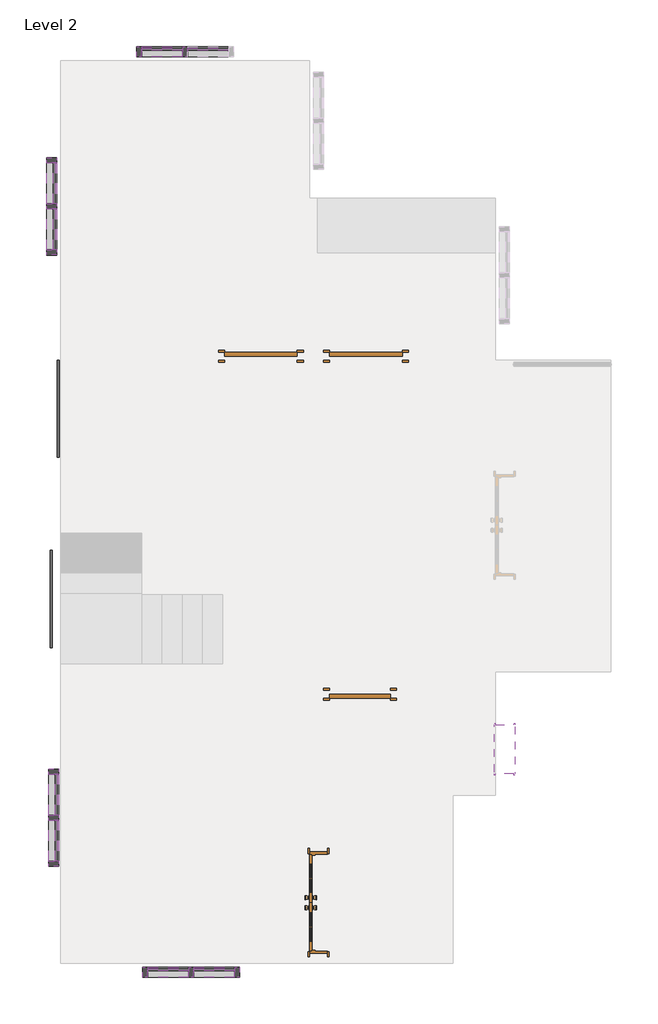
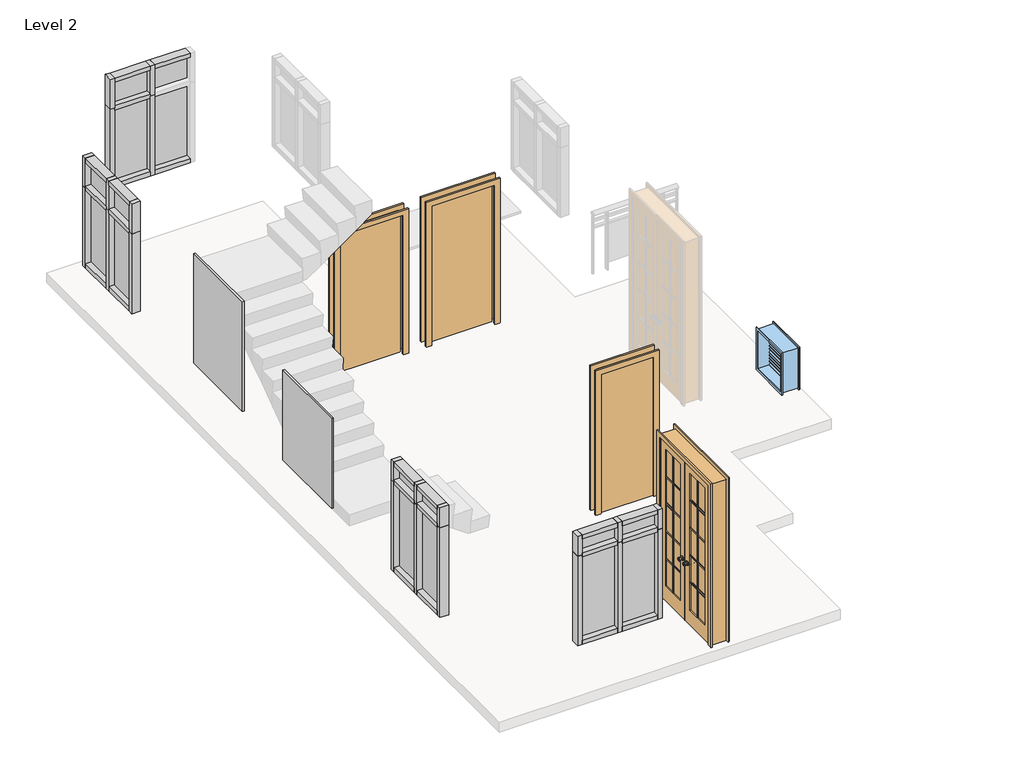
# One storey, part 1 of 2: 45 members, 18 plates, 4 doors, 1 window.
"""IFC4 building model written with IfcOpenShell, lengths in millimetres."""

from ifc_helpers import new_model, si_unit, origin, place, context, project, spatial, transform, mapped, element, save
from components import door_interior_double_full_glass_wood_4_x8_0c92ad92, door_270f2424, door_048588e9, door_310a3c6c, member_0b7646a3, member_2b49869a, member_aaa03826, member_ffd4c858, member_15823cb3, member_75074519, member_824a4a8d, member_75d1e245, member_3c3dc66a, member_c6627131, system_panel_glazed_d796fc41, system_panel_glazed_6374c067, system_panel_glazed_2596f6b1, system_panel_glazed_63160b6e, system_panel_glazed_45b685ca, system_panel_glazed_888d7767, window_f2d8fef0

model = new_model("IFC4")

# Units and contexts
model_context = context("Model", 3, world=origin())
ifc_project = project(units=[si_unit("LENGTHUNIT", "METRE", prefix="MILLI")], contexts=[model_context])

# Site, building, storey
site = spatial("IfcSite", under=ifc_project)
building = spatial("IfcBuilding", under=site)
storey = spatial("IfcBuildingStorey", under=building, Name="Level 2", Elevation=609.6)

# Doors
placement = place(None, origin())
door_interior_double_full_glass_wood_4_x8_shape = door_interior_double_full_glass_wood_4_x8_0c92ad92(model_context)
element("IfcDoor", 1, ObjectType="Door-Interior-Double-Full Glass-Wood : 4' x8'", at=placement, inside=storey, context=model_context, shape_type="MappedRepresentation", body=[
    mapped(door_interior_double_full_glass_wood_4_x8_shape, transform((-1598.3915653, -3197.0098448, 609.6), x_axis=(0.0, 1.0, 0.0), y_axis=(-1.0, 0.0, 0.0), z_axis=(0.0, 0.0, 1.0))),
])
door_shape = door_270f2424(model_context)
element("IfcDoor", 2, ObjectType="Single-Flush : 2'6\" x7'", at=placement, inside=storey, context=model_context, shape_type="MappedRepresentation", body=[
    mapped(door_shape, transform((-1074.5165653, -580.8142443, 609.6), x_axis=(-1.0, 0.0, 0.0), y_axis=(0.0, -1.0, 0.0), z_axis=(0.0, 0.0, 1.0))),
])
door_2_shape = door_048588e9(model_context)
element("IfcDoor", 3, ObjectType="Single-Flush : 36\" x 84\"", at=placement, inside=storey, context=model_context, shape_type="MappedRepresentation", body=[
    mapped(door_2_shape, transform((-2319.1165653, 3660.9857557, 609.6), x_axis=(1.0, 0.0, 0.0), y_axis=(0.0, 1.0, 0.0), z_axis=(0.0, 0.0, 1.0))),
])
door_3_shape = door_310a3c6c(model_context)
element("IfcDoor", 4, ObjectType="Single-Flush : 36\" x 84\"", at=placement, inside=storey, context=model_context, shape_type="MappedRepresentation", body=[
    mapped(door_3_shape, transform((-998.3165653, 3660.9857557, 609.6), x_axis=(-1.0, 0.0, 0.0), y_axis=(0.0, -1.0, 0.0), z_axis=(0.0, 0.0, 1.0))),
])

# Members
member_shape = member_0b7646a3(model_context)
element("IfcMember", 5, ObjectType="Rectangular Mullion : 2.5\" x 5\" rectangular", at=placement, inside=storey, context=model_context, shape_type="MappedRepresentation", body=[
    mapped(member_shape, transform((-4948.0165653, 4994.4857559, 3200.4), x_axis=(0.0, 0.0, 1.0), y_axis=(-1.0, 0.0, 0.0), z_axis=(0.0, -1.0, 0.0))),
])
element("IfcMember", 6, ObjectType="Rectangular Mullion : 2.5\" x 5\" rectangular", at=placement, inside=storey, context=model_context, shape_type="MappedRepresentation", body=[
    mapped(member_shape, transform((-4948.0165653, 5572.3357559, 3200.4), x_axis=(0.0, 0.0, 1.0), y_axis=(-1.0, 0.0, 0.0), z_axis=(0.0, -1.0, 0.0))),
])
element("IfcMember", 7, ObjectType="Rectangular Mullion : 2.5\" x 5\" rectangular", at=placement, inside=storey, context=model_context, shape_type="MappedRepresentation", body=[
    mapped(member_shape, transform((-2725.5165655, 7483.6857557, 3200.4), x_axis=(0.0, 0.0, 1.0), y_axis=(0.0, -1.0, 0.0), z_axis=(1.0, 0.0, 0.0))),
])
element("IfcMember", 8, ObjectType="Rectangular Mullion : 2.5\" x 5\" rectangular", at=placement, inside=storey, context=model_context, shape_type="MappedRepresentation", body=[
    mapped(member_shape, transform((-3303.3665655, 7483.6857557, 3200.4), x_axis=(0.0, 0.0, 1.0), y_axis=(0.0, -1.0, 0.0), z_axis=(1.0, 0.0, 0.0))),
])
element("IfcMember", 9, ObjectType="Rectangular Mullion : 2.5\" x 5\" rectangular", at=placement, inside=storey, context=model_context, shape_type="MappedRepresentation", body=[
    mapped(member_shape, transform((-4922.6165653, -2676.3142441, 3200.4), x_axis=(0.0, 0.0, 1.0), y_axis=(-1.0, 0.0, 0.0), z_axis=(0.0, -1.0, 0.0))),
])
element("IfcMember", 10, ObjectType="Rectangular Mullion : 2.5\" x 5\" rectangular", at=placement, inside=storey, context=model_context, shape_type="MappedRepresentation", body=[
    mapped(member_shape, transform((-4922.6165653, -2098.4642441, 3200.4), x_axis=(0.0, 0.0, 1.0), y_axis=(-1.0, 0.0, 0.0), z_axis=(0.0, -1.0, 0.0))),
])
element("IfcMember", 11, ObjectType="Rectangular Mullion : 2.5\" x 5\" rectangular", at=placement, inside=storey, context=model_context, shape_type="MappedRepresentation", body=[
    mapped(member_shape, transform((-2648.4534291, -4073.3142443, 3200.4), x_axis=(0.0, 0.0, 1.0), y_axis=(0.0, -1.0, 0.0), z_axis=(1.0, 0.0, 0.0))),
])
element("IfcMember", 12, ObjectType="Rectangular Mullion : 2.5\" x 5\" rectangular", at=placement, inside=storey, context=model_context, shape_type="MappedRepresentation", body=[
    mapped(member_shape, transform((-3226.3034291, -4073.3142443, 3200.4), x_axis=(0.0, 0.0, 1.0), y_axis=(0.0, -1.0, 0.0), z_axis=(1.0, 0.0, 0.0))),
])
element("IfcMember", 13, ObjectType="Rectangular Mullion : 2.5\" x 5\" rectangular", at=placement, inside=storey, context=model_context, shape_type="MappedRepresentation", body=[
    mapped(member_shape, transform((-4948.0165653, 6086.6857559, 1524.0), x_axis=(0.0, 0.0, -1.0), y_axis=(-1.0, 0.0, 0.0), z_axis=(0.0, 1.0, 0.0))),
])
element("IfcMember", 14, ObjectType="Rectangular Mullion : 2.5\" x 5\" rectangular", at=placement, inside=storey, context=model_context, shape_type="MappedRepresentation", body=[
    mapped(member_shape, transform((-4948.0165653, 5508.8357559, 1524.0), x_axis=(0.0, 0.0, -1.0), y_axis=(-1.0, 0.0, 0.0), z_axis=(0.0, 1.0, 0.0))),
])
element("IfcMember", 15, ObjectType="Rectangular Mullion : 2.5\" x 5\" rectangular", at=placement, inside=storey, context=model_context, shape_type="MappedRepresentation", body=[
    mapped(member_shape, transform((-3817.7165655, 7483.6857557, 1524.0), x_axis=(0.0, 0.0, -1.0), y_axis=(0.0, -1.0, 0.0), z_axis=(-1.0, 0.0, 0.0))),
])
element("IfcMember", 16, ObjectType="Rectangular Mullion : 2.5\" x 5\" rectangular", at=placement, inside=storey, context=model_context, shape_type="MappedRepresentation", body=[
    mapped(member_shape, transform((-3239.8665655, 7483.6857557, 1524.0), x_axis=(0.0, 0.0, -1.0), y_axis=(0.0, -1.0, 0.0), z_axis=(-1.0, 0.0, 0.0))),
])
element("IfcMember", 17, ObjectType="Rectangular Mullion : 2.5\" x 5\" rectangular", at=placement, inside=storey, context=model_context, shape_type="MappedRepresentation", body=[
    mapped(member_shape, transform((-4922.6165653, -1584.1142441, 1524.0), x_axis=(0.0, 0.0, -1.0), y_axis=(-1.0, 0.0, 0.0), z_axis=(0.0, 1.0, 0.0))),
])
element("IfcMember", 18, ObjectType="Rectangular Mullion : 2.5\" x 5\" rectangular", at=placement, inside=storey, context=model_context, shape_type="MappedRepresentation", body=[
    mapped(member_shape, transform((-4922.6165653, -2161.9642441, 1524.0), x_axis=(0.0, 0.0, -1.0), y_axis=(-1.0, 0.0, 0.0), z_axis=(0.0, 1.0, 0.0))),
])
element("IfcMember", 19, ObjectType="Rectangular Mullion : 2.5\" x 5\" rectangular", at=placement, inside=storey, context=model_context, shape_type="MappedRepresentation", body=[
    mapped(member_shape, transform((-3740.6534291, -4073.3142443, 1524.0), x_axis=(0.0, 0.0, -1.0), y_axis=(0.0, -1.0, 0.0), z_axis=(-1.0, 0.0, 0.0))),
])
element("IfcMember", 20, ObjectType="Rectangular Mullion : 2.5\" x 5\" rectangular", at=placement, inside=storey, context=model_context, shape_type="MappedRepresentation", body=[
    mapped(member_shape, transform((-3162.8034291, -4073.3142443, 1524.0), x_axis=(0.0, 0.0, -1.0), y_axis=(0.0, -1.0, 0.0), z_axis=(-1.0, 0.0, 0.0))),
])
member_2_shape = member_2b49869a(model_context)
element("IfcMember", 21, ObjectType="Rectangular Mullion : 2.5\" x 5\" rectangular", at=placement, inside=storey, context=model_context, shape_type="MappedRepresentation", body=[
    mapped(member_2_shape, transform((-4948.0165653, 5540.5857559, 1524.0), x_axis=(0.0, -1.0, 0.0), y_axis=(-1.0, 0.0, 0.0), z_axis=(0.0, 0.0, -1.0))),
])
element("IfcMember", 22, ObjectType="Rectangular Mullion : 2.5\" x 5\" rectangular", at=placement, inside=storey, context=model_context, shape_type="MappedRepresentation", body=[
    mapped(member_2_shape, transform((-3271.6165655, 7483.6857557, 1524.0), x_axis=(1.0, 0.0, 0.0), y_axis=(0.0, -1.0, 0.0), z_axis=(0.0, 0.0, -1.0))),
])
member_3_shape = member_aaa03826(model_context)
element("IfcMember", 23, ObjectType="Rectangular Mullion : 2.5\" x 5\" rectangular", at=placement, inside=storey, context=model_context, shape_type="MappedRepresentation", body=[
    mapped(member_3_shape, transform((-4948.0165653, 5572.3357559, 2743.2), x_axis=(0.0, 0.0, 1.0), y_axis=(-1.0, 0.0, 0.0), z_axis=(0.0, -1.0, 0.0))),
])
element("IfcMember", 24, ObjectType="Rectangular Mullion : 2.5\" x 5\" rectangular", at=placement, inside=storey, context=model_context, shape_type="MappedRepresentation", body=[
    mapped(member_3_shape, transform((-4948.0165653, 4994.4857559, 2743.2), x_axis=(0.0, 0.0, 1.0), y_axis=(-1.0, 0.0, 0.0), z_axis=(0.0, -1.0, 0.0))),
])
element("IfcMember", 25, ObjectType="Rectangular Mullion : 2.5\" x 5\" rectangular", at=placement, inside=storey, context=model_context, shape_type="MappedRepresentation", body=[
    mapped(member_3_shape, transform((-3303.3665655, 7483.6857557, 2743.2), x_axis=(0.0, 0.0, 1.0), y_axis=(0.0, -1.0, 0.0), z_axis=(1.0, 0.0, 0.0))),
])
element("IfcMember", 26, ObjectType="Rectangular Mullion : 2.5\" x 5\" rectangular", at=placement, inside=storey, context=model_context, shape_type="MappedRepresentation", body=[
    mapped(member_3_shape, transform((-4922.6165653, -2098.4642441, 2895.6), x_axis=(0.0, 0.0, 1.0), y_axis=(-1.0, 0.0, 0.0), z_axis=(0.0, -1.0, 0.0))),
])
element("IfcMember", 27, ObjectType="Rectangular Mullion : 2.5\" x 5\" rectangular", at=placement, inside=storey, context=model_context, shape_type="MappedRepresentation", body=[
    mapped(member_3_shape, transform((-4922.6165653, -2676.3142441, 2895.6), x_axis=(0.0, 0.0, 1.0), y_axis=(-1.0, 0.0, 0.0), z_axis=(0.0, -1.0, 0.0))),
])
element("IfcMember", 28, ObjectType="Rectangular Mullion : 2.5\" x 5\" rectangular", at=placement, inside=storey, context=model_context, shape_type="MappedRepresentation", body=[
    mapped(member_3_shape, transform((-3226.3034291, -4073.3142443, 2895.6), x_axis=(0.0, 0.0, 1.0), y_axis=(0.0, -1.0, 0.0), z_axis=(1.0, 0.0, 0.0))),
])
element("IfcMember", 29, ObjectType="Rectangular Mullion : 2.5\" x 5\" rectangular", at=placement, inside=storey, context=model_context, shape_type="MappedRepresentation", body=[
    mapped(member_3_shape, transform((-2648.4534291, -4073.3142443, 2895.6), x_axis=(0.0, 0.0, 1.0), y_axis=(0.0, -1.0, 0.0), z_axis=(1.0, 0.0, 0.0))),
])
member_4_shape = member_ffd4c858(model_context)
element("IfcMember", 30, ObjectType="Rectangular Mullion : 2.5\" x 5\" rectangular", at=placement, inside=storey, context=model_context, shape_type="MappedRepresentation", body=[
    mapped(member_4_shape, transform((-4948.0165653, 5540.5857559, 2743.2), x_axis=(0.0, -1.0, 0.0), y_axis=(-1.0, 0.0, 0.0), z_axis=(0.0, 0.0, -1.0))),
])
element("IfcMember", 31, ObjectType="Rectangular Mullion : 2.5\" x 5\" rectangular", at=placement, inside=storey, context=model_context, shape_type="MappedRepresentation", body=[
    mapped(member_4_shape, transform((-3271.6165655, 7483.6857557, 2743.2), x_axis=(1.0, 0.0, 0.0), y_axis=(0.0, -1.0, 0.0), z_axis=(0.0, 0.0, -1.0))),
])
member_5_shape = member_15823cb3(model_context)
element("IfcMember", 32, ObjectType="Rectangular Mullion : 2.5\" x 5\" rectangular", at=placement, inside=storey, context=model_context, shape_type="MappedRepresentation", body=[
    mapped(member_5_shape, transform((-4948.0165653, 6150.1857559, 3200.4), x_axis=(0.0, 1.0, 0.0), y_axis=(-1.0, 0.0, 0.0), z_axis=(0.0, 0.0, 1.0))),
])
element("IfcMember", 33, ObjectType="Rectangular Mullion : 2.5\" x 5\" rectangular", at=placement, inside=storey, context=model_context, shape_type="MappedRepresentation", body=[
    mapped(member_5_shape, transform((-3881.2165655, 7483.6857557, 3200.4), x_axis=(-1.0, 0.0, 0.0), y_axis=(0.0, -1.0, 0.0), z_axis=(0.0, 0.0, 1.0))),
])
member_6_shape = member_75074519(model_context)
element("IfcMember", 34, ObjectType="Rectangular Mullion : 2.5\" x 5\" rectangular", at=placement, inside=storey, context=model_context, shape_type="MappedRepresentation", body=[
    mapped(member_6_shape, transform((-4948.0165653, 4930.9857559, 1524.0), x_axis=(0.0, -1.0, 0.0), y_axis=(-1.0, 0.0, 0.0), z_axis=(0.0, 0.0, -1.0))),
])
element("IfcMember", 35, ObjectType="Rectangular Mullion : 2.5\" x 5\" rectangular", at=placement, inside=storey, context=model_context, shape_type="MappedRepresentation", body=[
    mapped(member_5_shape, transform((-4948.0165653, 4930.9857559, 2743.2), x_axis=(0.0, -1.0, 0.0), y_axis=(-1.0, 0.0, 0.0), z_axis=(0.0, 0.0, -1.0))),
])
element("IfcMember", 36, ObjectType="Rectangular Mullion : 2.5\" x 5\" rectangular", at=placement, inside=storey, context=model_context, shape_type="MappedRepresentation", body=[
    mapped(member_6_shape, transform((-4948.0165653, 6150.1857559, 2743.2), x_axis=(0.0, 1.0, 0.0), y_axis=(-1.0, 0.0, 0.0), z_axis=(0.0, 0.0, 1.0))),
])
element("IfcMember", 37, ObjectType="Rectangular Mullion : 2.5\" x 5\" rectangular", at=placement, inside=storey, context=model_context, shape_type="MappedRepresentation", body=[
    mapped(member_6_shape, transform((-3881.2165655, 7483.6857557, 2743.2), x_axis=(-1.0, 0.0, 0.0), y_axis=(0.0, -1.0, 0.0), z_axis=(0.0, 0.0, 1.0))),
])
member_7_shape = member_824a4a8d(model_context)
element("IfcMember", 38, ObjectType="Rectangular Mullion : 2.5\" x 5\" rectangular", at=placement, inside=storey, context=model_context, shape_type="MappedRepresentation", body=[
    mapped(member_7_shape, transform((-4922.6165653, -2130.2142441, 1524.0), x_axis=(0.0, -1.0, 0.0), y_axis=(-1.0, 0.0, 0.0), z_axis=(0.0, 0.0, -1.0))),
])
element("IfcMember", 39, ObjectType="Rectangular Mullion : 2.5\" x 5\" rectangular", at=placement, inside=storey, context=model_context, shape_type="MappedRepresentation", body=[
    mapped(member_7_shape, transform((-3194.5534291, -4073.3142443, 1524.0), x_axis=(1.0, 0.0, 0.0), y_axis=(0.0, -1.0, 0.0), z_axis=(0.0, 0.0, -1.0))),
])
member_8_shape = member_75d1e245(model_context)
element("IfcMember", 40, ObjectType="Rectangular Mullion : 2.5\" x 5\" rectangular", at=placement, inside=storey, context=model_context, shape_type="MappedRepresentation", body=[
    mapped(member_8_shape, transform((-4922.6165653, -2130.2142441, 2895.6), x_axis=(0.0, -1.0, 0.0), y_axis=(-1.0, 0.0, 0.0), z_axis=(0.0, 0.0, -1.0))),
])
element("IfcMember", 41, ObjectType="Rectangular Mullion : 2.5\" x 5\" rectangular", at=placement, inside=storey, context=model_context, shape_type="MappedRepresentation", body=[
    mapped(member_8_shape, transform((-3194.5534291, -4073.3142443, 2895.6), x_axis=(1.0, 0.0, 0.0), y_axis=(0.0, -1.0, 0.0), z_axis=(0.0, 0.0, -1.0))),
])
member_9_shape = member_3c3dc66a(model_context)
element("IfcMember", 42, ObjectType="Rectangular Mullion : 2.5\" x 5\" rectangular", at=placement, inside=storey, context=model_context, shape_type="MappedRepresentation", body=[
    mapped(member_9_shape, transform((-4922.6165653, -1520.6142441, 3200.4), x_axis=(0.0, 1.0, 0.0), y_axis=(-1.0, 0.0, 0.0), z_axis=(0.0, 0.0, 1.0))),
])
element("IfcMember", 43, ObjectType="Rectangular Mullion : 2.5\" x 5\" rectangular", at=placement, inside=storey, context=model_context, shape_type="MappedRepresentation", body=[
    mapped(member_9_shape, transform((-3804.1534291, -4073.3142443, 3200.4), x_axis=(-1.0, 0.0, 0.0), y_axis=(0.0, -1.0, 0.0), z_axis=(0.0, 0.0, 1.0))),
])
member_10_shape = member_c6627131(model_context)
element("IfcMember", 44, ObjectType="Rectangular Mullion : 2.5\" x 5\" rectangular", at=placement, inside=storey, context=model_context, shape_type="MappedRepresentation", body=[
    mapped(member_10_shape, transform((-4922.6165653, -2739.8142441, 1524.0), x_axis=(0.0, -1.0, 0.0), y_axis=(-1.0, 0.0, 0.0), z_axis=(0.0, 0.0, -1.0))),
])
element("IfcMember", 45, ObjectType="Rectangular Mullion : 2.5\" x 5\" rectangular", at=placement, inside=storey, context=model_context, shape_type="MappedRepresentation", body=[
    mapped(member_10_shape, transform((-2584.9534291, -4073.3142443, 1524.0), x_axis=(1.0, 0.0, 0.0), y_axis=(0.0, -1.0, 0.0), z_axis=(0.0, 0.0, -1.0))),
])
element("IfcMember", 46, ObjectType="Rectangular Mullion : 2.5\" x 5\" rectangular", at=placement, inside=storey, context=model_context, shape_type="MappedRepresentation", body=[
    mapped(member_9_shape, transform((-4922.6165653, -2739.8142441, 2895.6), x_axis=(0.0, -1.0, 0.0), y_axis=(-1.0, 0.0, 0.0), z_axis=(0.0, 0.0, -1.0))),
])
element("IfcMember", 47, ObjectType="Rectangular Mullion : 2.5\" x 5\" rectangular", at=placement, inside=storey, context=model_context, shape_type="MappedRepresentation", body=[
    mapped(member_9_shape, transform((-2584.9534291, -4073.3142443, 2895.6), x_axis=(1.0, 0.0, 0.0), y_axis=(0.0, -1.0, 0.0), z_axis=(0.0, 0.0, -1.0))),
])
element("IfcMember", 48, ObjectType="Rectangular Mullion : 2.5\" x 5\" rectangular", at=placement, inside=storey, context=model_context, shape_type="MappedRepresentation", body=[
    mapped(member_10_shape, transform((-4922.6165653, -1520.6142441, 2895.6), x_axis=(0.0, 1.0, 0.0), y_axis=(-1.0, 0.0, 0.0), z_axis=(0.0, 0.0, 1.0))),
])
element("IfcMember", 49, ObjectType="Rectangular Mullion : 2.5\" x 5\" rectangular", at=placement, inside=storey, context=model_context, shape_type="MappedRepresentation", body=[
    mapped(member_10_shape, transform((-3804.1534291, -4073.3142443, 2895.6), x_axis=(-1.0, 0.0, 0.0), y_axis=(0.0, -1.0, 0.0), z_axis=(0.0, 0.0, 1.0))),
])

# Plates
system_panel_glazed_shape = system_panel_glazed_d796fc41(model_context)
element("IfcPlate", 50, ObjectType="System Panel : Glazed", at=placement, inside=storey, context=model_context, shape_type="MappedRepresentation", body=[
    mapped(system_panel_glazed_shape, transform((-4948.0165653, 5829.5107559, 1587.5), x_axis=(0.0, -1.0, 0.0), y_axis=(1.0, 0.0, 0.0), z_axis=(0.0, 0.0, 1.0))),
])
element("IfcPlate", 51, ObjectType="System Panel : Glazed", at=placement, inside=storey, context=model_context, shape_type="MappedRepresentation", body=[
    mapped(system_panel_glazed_shape, transform((-4948.0165653, 5251.6607559, 1587.5), x_axis=(0.0, -1.0, 0.0), y_axis=(1.0, 0.0, 0.0), z_axis=(0.0, 0.0, 1.0))),
])
element("IfcPlate", 52, ObjectType="System Panel : Glazed", at=placement, inside=storey, context=model_context, shape_type="MappedRepresentation", body=[
    mapped(system_panel_glazed_shape, transform((-3560.5415655, 7483.6857557, 1587.5), x_axis=(1.0, 0.0, 0.0), y_axis=(0.0, 1.0, 0.0), z_axis=(0.0, 0.0, 1.0))),
])
element("IfcPlate", 53, ObjectType="System Panel : Glazed", at=placement, inside=storey, context=model_context, shape_type="MappedRepresentation", body=[
    mapped(system_panel_glazed_shape, transform((-2982.6915655, 7483.6857557, 1587.5), x_axis=(1.0, 0.0, 0.0), y_axis=(0.0, 1.0, 0.0), z_axis=(0.0, 0.0, 1.0))),
])
system_panel_glazed_2_shape = system_panel_glazed_6374c067(model_context)
element("IfcPlate", 54, ObjectType="System Panel : Glazed", at=placement, inside=storey, context=model_context, shape_type="MappedRepresentation", body=[
    mapped(system_panel_glazed_2_shape, transform((-4948.0165653, 5829.5107559, 2774.95), x_axis=(0.0, -1.0, 0.0), y_axis=(1.0, 0.0, 0.0), z_axis=(0.0, 0.0, 1.0))),
])
element("IfcPlate", 55, ObjectType="System Panel : Glazed", at=placement, inside=storey, context=model_context, shape_type="MappedRepresentation", body=[
    mapped(system_panel_glazed_2_shape, transform((-4948.0165653, 5251.6607559, 2774.95), x_axis=(0.0, -1.0, 0.0), y_axis=(1.0, 0.0, 0.0), z_axis=(0.0, 0.0, 1.0))),
])
element("IfcPlate", 56, ObjectType="System Panel : Glazed", at=placement, inside=storey, context=model_context, shape_type="MappedRepresentation", body=[
    mapped(system_panel_glazed_2_shape, transform((-3560.5415655, 7483.6857557, 2774.95), x_axis=(1.0, 0.0, 0.0), y_axis=(0.0, 1.0, 0.0), z_axis=(0.0, 0.0, 1.0))),
])
element("IfcPlate", 57, ObjectType="System Panel : Glazed", at=placement, inside=storey, context=model_context, shape_type="MappedRepresentation", body=[
    mapped(system_panel_glazed_2_shape, transform((-2982.6915655, 7483.6857557, 2774.95), x_axis=(1.0, 0.0, 0.0), y_axis=(0.0, 1.0, 0.0), z_axis=(0.0, 0.0, 1.0))),
])
system_panel_glazed_3_shape = system_panel_glazed_2596f6b1(model_context)
element("IfcPlate", 58, ObjectType="System Panel : Glazed", at=placement, inside=storey, context=model_context, shape_type="MappedRepresentation", body=[
    mapped(system_panel_glazed_3_shape, transform((-3483.4784291, -4073.3142443, 1587.5), x_axis=(1.0, 0.0, 0.0), y_axis=(0.0, 1.0, 0.0), z_axis=(0.0, 0.0, 1.0))),
])
element("IfcPlate", 59, ObjectType="System Panel : Glazed", at=placement, inside=storey, context=model_context, shape_type="MappedRepresentation", body=[
    mapped(system_panel_glazed_3_shape, transform((-4922.6165653, -1841.2892441, 1587.5), x_axis=(0.0, -1.0, 0.0), y_axis=(1.0, 0.0, 0.0), z_axis=(0.0, 0.0, 1.0))),
])
element("IfcPlate", 60, ObjectType="System Panel : Glazed", at=placement, inside=storey, context=model_context, shape_type="MappedRepresentation", body=[
    mapped(system_panel_glazed_3_shape, transform((-4922.6165653, -2419.1392441, 1587.5), x_axis=(0.0, -1.0, 0.0), y_axis=(1.0, 0.0, 0.0), z_axis=(0.0, 0.0, 1.0))),
])
element("IfcPlate", 61, ObjectType="System Panel : Glazed", at=placement, inside=storey, context=model_context, shape_type="MappedRepresentation", body=[
    mapped(system_panel_glazed_3_shape, transform((-2905.6284291, -4073.3142443, 1587.5), x_axis=(1.0, 0.0, 0.0), y_axis=(0.0, 1.0, 0.0), z_axis=(0.0, 0.0, 1.0))),
])
system_panel_glazed_4_shape = system_panel_glazed_63160b6e(model_context)
element("IfcPlate", 62, ObjectType="System Panel : Glazed", at=placement, inside=storey, context=model_context, shape_type="MappedRepresentation", body=[
    mapped(system_panel_glazed_4_shape, transform((-4922.6165653, -1841.2892441, 2927.35), x_axis=(0.0, -1.0, 0.0), y_axis=(1.0, 0.0, 0.0), z_axis=(0.0, 0.0, 1.0))),
])
element("IfcPlate", 63, ObjectType="System Panel : Glazed", at=placement, inside=storey, context=model_context, shape_type="MappedRepresentation", body=[
    mapped(system_panel_glazed_4_shape, transform((-4922.6165653, -2419.1392441, 2927.35), x_axis=(0.0, -1.0, 0.0), y_axis=(1.0, 0.0, 0.0), z_axis=(0.0, 0.0, 1.0))),
])
element("IfcPlate", 64, ObjectType="System Panel : Glazed", at=placement, inside=storey, context=model_context, shape_type="MappedRepresentation", body=[
    mapped(system_panel_glazed_4_shape, transform((-3483.4784291, -4073.3142443, 2927.35), x_axis=(1.0, 0.0, 0.0), y_axis=(0.0, 1.0, 0.0), z_axis=(0.0, 0.0, 1.0))),
])
element("IfcPlate", 65, ObjectType="System Panel : Glazed", at=placement, inside=storey, context=model_context, shape_type="MappedRepresentation", body=[
    mapped(system_panel_glazed_4_shape, transform((-2905.6284291, -4073.3142443, 2927.35), x_axis=(1.0, 0.0, 0.0), y_axis=(0.0, 1.0, 0.0), z_axis=(0.0, 0.0, 1.0))),
])
system_panel_glazed_5_shape = system_panel_glazed_45b685ca(model_context)
element("IfcPlate", 66, ObjectType="System Panel : Glazed", at=placement, inside=storey, context=model_context, shape_type="MappedRepresentation", body=[
    mapped(system_panel_glazed_5_shape, transform((-4922.6165653, 612.9857557, 1524.0), x_axis=(0.0, 1.0, 0.0), y_axis=(-1.0, 0.0, 0.0), z_axis=(0.0, 0.0, 1.0))),
])
system_panel_glazed_6_shape = system_panel_glazed_888d7767(model_context)
element("IfcPlate", 67, ObjectType="System Panel : Glazed", at=placement, inside=storey, context=model_context, shape_type="MappedRepresentation", body=[
    mapped(system_panel_glazed_6_shape, transform((-4897.2165653, 3000.5857558, 1524.0), x_axis=(0.0, -1.0, 0.0), y_axis=(1.0, 0.0, 0.0), z_axis=(0.0, 0.0, 1.0))),
])

# Window
window_shape = window_f2d8fef0(model_context)
element("IfcWindow", 68, ObjectType="Window-Louvers : 24\" x 24\"", at=placement, inside=storey, context=model_context, shape_type="MappedRepresentation", body=[
    mapped(window_shape, transform((747.9334347, -1272.9642443, 1371.6), x_axis=(0.0, -1.0, 0.0), y_axis=(1.0, 0.0, 0.0), z_axis=(0.0, 0.0, 1.0))),
])

save(model, "model.ifc")

# Revit data of these elements
# Type "Door-Interior-Double-Full Glass-Wood : 4' x8'"
#   Type Mark = "14"
#   Assembly Code = "C1020300"
#   Analytic Construction = "French door, wood frame with single glass"
#   Top Rail = 0' - 4 11/16"
#   Thickness = 0' - 1 3/8"
#   Thermal Resistance (R) = 1.0696 (h·ft²·°F)/BTU
#   Swing Angle [instance default] = 90.00°
#   Stiles = 0' - 4 3/4"
#   Rough Width = 4' - 2"
#   Rough Height = 8' - 1"
#   Panel Width = 2' - 0"
#   Height = 8' - 0"
#   Width = 4' - 0"
#   Heat Transfer Coefficient (U) = 0.9350 BTU/(h·ft²·°F)
#   Bottom Rail = 0' - 9 1/8"
#   Show Grill [instance default] = yes
#   Trim Material = Cherry
#   Panel Material = Cherry
#   Frame Material = Cherry
#   Door Handle Material = Aluminum
#   Visual Light Transmittance = 0
#   Solar Heat Gain Coefficient = 0
#   Wall Closure = (empty or 0)
#   Function = (empty or 0)
# Type "Single-Flush : 2'6\" x7'"
#   Type Mark = "15"
#   Construction Type Id = "MDOOR"
#   Assembly Code = "C1020"
#   Analytic Construction = "Metal"
#   Thickness = 0' - 2"
#   Heat Transfer Coefficient (U) = 0.651978 BTU/(h·ft²·°F)
#   Height = 7' - 0"
#   Trim Projection Ext = 0' - 1"
#   Trim Projection Int = 0' - 1"
#   Trim Width = 0' - 3"
#   Width = 2' - 6"
#   Define Thermal Properties by = 1
#   Door Material = Door - Panel
#   Frame Material = Door - Frame
#   Visual Light Transmittance = 0
#   Solar Heat Gain Coefficient = 0
#   Function = (empty or 0)
#   Wall Closure = (empty or 0)
# Type "Single-Flush : 36\" x 84\""
#   Type Mark = "5"
#   Construction Type Id = "MDOOR"
#   Assembly Code = "C1020"
#   Analytic Construction = "Metal"
#   Thickness = 0' - 2"
#   Heat Transfer Coefficient (U) = 0.651978 BTU/(h·ft²·°F)
#   Height = 7' - 0"
#   Trim Projection Ext = 0' - 1"
#   Trim Projection Int = 0' - 1"
#   Trim Width = 0' - 3"
#   Width = 3' - 0"
#   Define Thermal Properties by = 1
#   Define Thermal Properties by = 1
#   Door Material = Door - Panel
#   Frame Material = Door - Frame
#   Visual Light Transmittance = 0
#   Solar Heat Gain Coefficient = 0
#   Function = (empty or 0)
#   Wall Closure = (empty or 0)
# Type "Rectangular Mullion : 2.5\" x 5\" rectangular"
#   built-in parameter 1007304 = 0.416667 (stored number, unit not read)
#   built-in parameter 1007301 = 0.104167 (stored number, unit not read)
#   built-in parameter 1007300 = 0.104167 (stored number, unit not read)
# Type "System Panel : Glazed"
#   Construction Type Id = "GSP4R"
#   Analytic Construction = "1/8 in Pilkington single glazing"
#   Visual Light Transmittance = 0.9
#   Solar Heat Gain Coefficient = 0.86
#   Heat Transfer Coefficient (U) = 1.18115 BTU/(h·ft²·°F)
#   Define Thermal Properties by = 1
# Type "Window-Louvers : 24\" x 24\""
#   Type Mark = "18"
#   Construction Type Id = "GSP4R"
#   Assembly Code = "B20"
#   Analytic Construction = "1/8 in Pilkington single glazing"
#   Visual Light Transmittance = 0.9
#   Thermal Resistance (R) = 1.53941 (h·ft²·°F)/BTU
#   Solar Heat Gain Coefficient = 0.78
#   Max Height = 1' - 11.74264"
#   Height = 2' - 0"
#   Heat Transfer Coefficient (U) = 0.6496 BTU/(h·ft²·°F)
#   Blade Width [instance default] = 1' - 10 1/2"
#   Blade Vertical Thickness = 0' - 0.35355"
#   Blade Thickness = 0' - 0 1/4"
#   Blade Spacing = 0' - 1 1/2"
#   Blade Height = 0' - 1.85355"
#   Blade Depth = 0' - 3"
#   Blade Angle = 45.00°
#   Default Sill Height = 3' - 0"
#   Trim Projection_Exterior = 0' - 0 1/2"
#   Trim Projection_Interior = 0' - 0 1/2"
#   Trim Width_Exterior = 0' - 1 1/2"
#   Trim Width_Interior = 0' - 1 1/2"
#   Width = 2' - 0"
#   Max Blade Count = 12
#   Define Thermal Properties by = 1
#   Blade Count = 12
#   Frame Material = Birch
#   Louver Material = Birch
#   Trim Exterior Material = Birch
#   Trim Interior Material = Birch
#   Wall Closure = (empty or 0)
# Element 1 (IfcDoor, "Door-Interior-Double-Full Glass-Wood : 4' x8'")
#   Swing Angle = 45.00°
#   Show Grill = yes
#   Phase Created = New Construction
#   Materials on its faces: "Cherry", "Aluminum", "Glass"
# Element 2 (IfcDoor, "Single-Flush : 2'6\" x7'")
#   Phase Created = New Construction
#   Materials on its faces: "Door - Frame", "Door - Panel"
# Elements 3, 4 (IfcDoor, "Single-Flush : 36\" x 84\"")
#   Phase Created = New Construction
#   Materials on its faces: "Door - Frame", "Door - Panel"
# Elements 5, 6, 7, 8, 9, 10, 11, 12, 13, 14, 15, 16, 17, 18, 19, 20, 21, 22, 23, 24, 25, 26, 27, 28, 29, 30, 31, 32, 33, 34, 35, 36, 37, 38, 39, 40, 41, 42, 43, 44, 45, 46, 47, 48, 49 (IfcMember, "Rectangular Mullion : 2.5\" x 5\" rectangular")
#   Phase Created = New Construction
#   Materials on its faces: "Aluminum"
# Elements 50, 51, 52, 53, 54, 55, 56, 57, 58, 59, 60, 61, 62, 63, 64, 65, 66, 67 (IfcPlate, "System Panel : Glazed")
#   Phase Created = New Construction
#   Materials on its faces: "Glass"
# Element 68 (IfcWindow, "Window-Louvers : 24\" x 24\"")
#   Mark = "3"
#   Blade Width = 1' - 10 1/2"
#   Phase Created = New Construction
#   Materials on its faces: "Birch"
# Materials
#   "Cherry": class "Wood", colour RGB 226 177 128, transparency 0, Description = "Prunus Serotina", Cost = 0
#   "Aluminum": class "Metal", colour RGB 247 247 247, transparency 0, Description = "Aluminum 6061", Cost = 0
#   "Door - Panel": class "Wood", colour RGB 210 159 95, transparency 0, Cost = 0
#   "Door - Frame": colour RGB 118 70 51, transparency 0, Cost = 0
#   "Birch": class "Wood", colour RGB 224 178 126, transparency 0, Description = "Betula Alleghaniensis", Cost = 0
#   "Glass": class "Glass", colour RGB 0 128 192, transparency 0.75, Description = "Soda Lime Glass", Cost = 0
